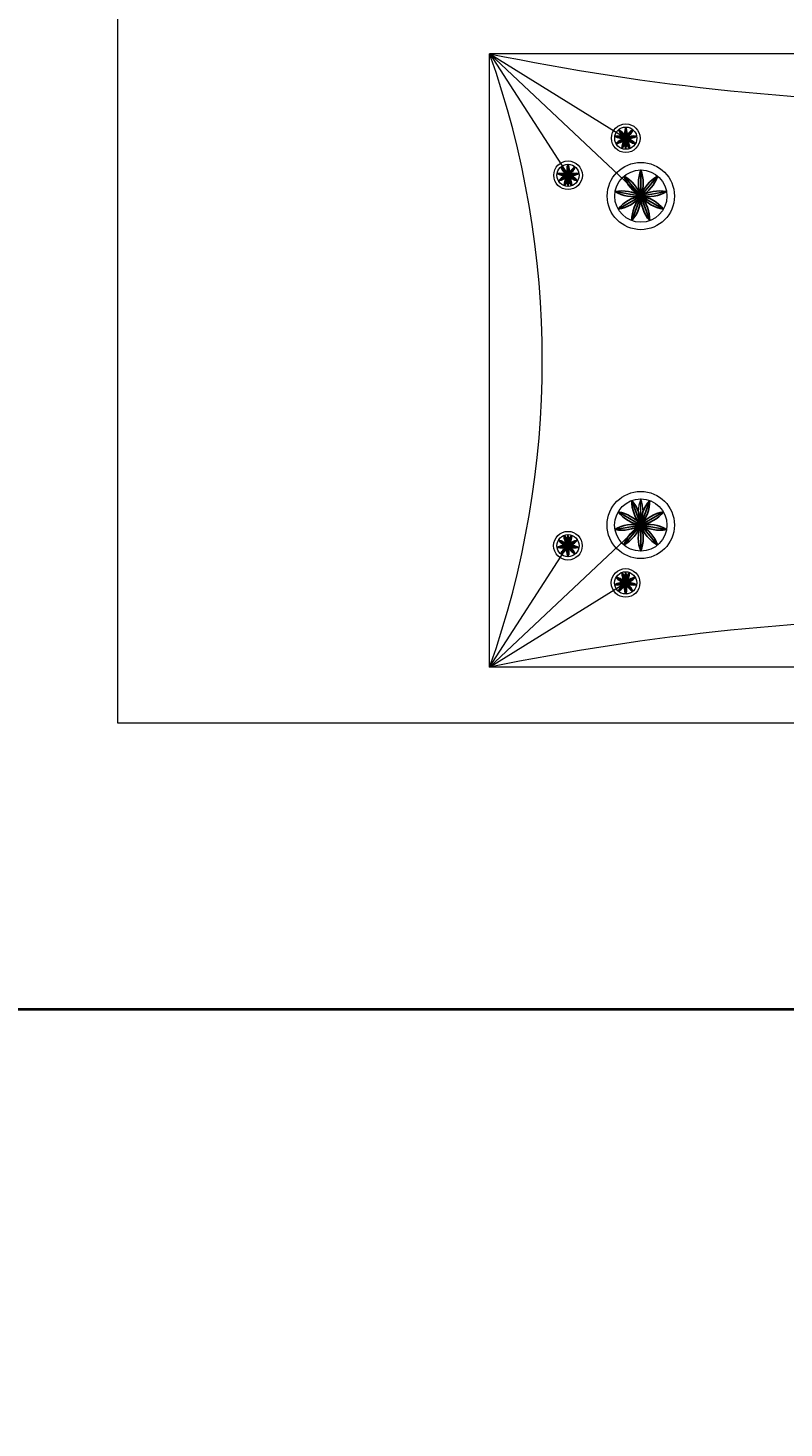
# Model space of a CAD drawing. Units: inches. Extents: x -46 to 1145, y -527 to 760.
# Tile 25 of 57: x 47 to 63, y 222 to 252. Entities that reach past the tile are written whole.
import ezdxf

# ---------------------------------------------------------------- set-up
doc = ezdxf.new("R2010")
doc.units = ezdxf.units.IN
doc.header["$MEASUREMENT"] = 0
for name, color, linetype, lineweight in [('A-ANNO-DIMS', 2, 'Continuous', 18), ('A-FURN', 2, 'Continuous', 13), ('WALLS', 4, 'Continuous', 40)]:
    doc.layers.add(name, color=color, linetype=linetype, lineweight=lineweight)
doc.layers.add('LT', color=9, linetype='Continuous')
doc.styles.get("Standard").update_dxf_attribs({"font": 'arial.ttf'})
doc.dimstyles.get("Standard").update_dxf_attribs({"dimtxt": 0.18, "dimasz": 0.18, "dimexe": 0.18, "dimexo": 0.0625, "dimgap": 0.09, "dimtad": 0, "dimtih": 1, "dimtoh": 1, "dimdec": 0, "dimzin": 0, "dimdsep": 46, "dimlunit": 3, "dimtxsty": 'Standard', "dimcen": 0.09, "dimadec": 0, "dimazin": 0, "dimtfac": 1, "dimtdec": 0, "dimtofl": 0, "dimtmove": 0, "dimatfit": 3, "dimfxl": 1, "dimtolj": 1, "dimtzin": 0, "dimarcsym": 0})

# ---------------------------------------------------------------- blocks, each defined once
blk = doc.blocks.new('*U58')
at = {"layer": 'LT'}
blk.add_line((0, 0.281), (0, -0.281), dxfattribs=at)
for centre, start, end in [((0.734, 0), 159.0676, 200.9324), ((-0.734, 0), 339.0676, 20.9324)]:
    blk.add_arc(centre, 0.786, start, end, dxfattribs=at)
blk = doc.blocks.new('*U59')
at = {"layer": 'LT', "transparency": 16777216}
blk.add_blockref('*U58', (609.936, 444.026), dxfattribs=at)
for p, rotation in [((609.756, 443.96), 40.00000000000002), ((610.117, 443.96), 320), ((609.659, 443.794), 80.00000000000001), ((609.693, 443.605), 120), ((609.84, 443.481), 160), ((610.032, 443.481), 200), ((610.179, 443.605), 240), ((610.213, 443.794), 280)]:
    blk.add_blockref('*U58', p, dxfattribs=dict(at, rotation=rotation))
blk = doc.blocks.new('*U60')
at = {"layer": 'LT'}
blk.add_line((0, 0.12), (0, -0.12), dxfattribs=at)
for centre, start, end in [((0.313, 0), 159.0676, 200.9324), ((-0.313, 0), 339.0676, 20.9324)]:
    blk.add_arc(centre, 0.335, start, end, dxfattribs=at)
blk = doc.blocks.new('*U61')
at = {"layer": 'LT', "transparency": 16777216}
for p, rotation in [((259.495, 188.896), 80.00000000000001), ((259.509, 188.816), 120), ((259.536, 188.967), 40), ((259.572, 188.763), 160), ((259.654, 188.763), 200), ((259.69, 188.967), 320), ((259.716, 188.816), 240), ((259.731, 188.896), 280)]:
    blk.add_blockref('*U60', p, dxfattribs=dict(at, rotation=rotation))
blk.add_blockref('*U60', (259.613, 188.995), dxfattribs=at)
blk = doc.blocks.new('*U62')
at = {"layer": 'LT'}
blk.add_line((0, 0.12), (0, -0.12), dxfattribs=at)
for centre, start, end in [((0.313, 0), 159.0676, 200.9324), ((-0.313, 0), 339.0676, 20.9324)]:
    blk.add_arc(centre, 0.335, start, end, dxfattribs=at)
blk = doc.blocks.new('*U63')
at = {"layer": 'LT', "transparency": 16777216}
for p, rotation in [((259.495, 188.896), 80.00000000000001), ((259.509, 188.816), 120), ((259.536, 188.967), 40), ((259.572, 188.763), 160), ((259.654, 188.763), 200), ((259.69, 188.967), 320), ((259.716, 188.816), 240), ((259.731, 188.896), 280)]:
    blk.add_blockref('*U62', p, dxfattribs=dict(at, rotation=rotation))
blk.add_blockref('*U62', (259.613, 188.995), dxfattribs=at)
blk = doc.blocks.new('*U70')
at = {"layer": 'LT'}
blk.add_line((0, 0.281), (0, -0.281), dxfattribs=at)
for centre, start, end in [((0.734, 0), 159.0676, 200.9324), ((-0.734, 0), 339.0676, 20.9324)]:
    blk.add_arc(centre, 0.786, start, end, dxfattribs=at)
blk = doc.blocks.new('*U71')
at = {"layer": 'LT', "transparency": 16777216}
blk.add_blockref('*U70', (609.936, 444.026), dxfattribs=at)
for p, rotation in [((609.756, 443.96), 40.00000000000002), ((610.117, 443.96), 320), ((609.659, 443.794), 80.00000000000001), ((609.693, 443.605), 120), ((609.84, 443.481), 160), ((610.032, 443.481), 200), ((610.179, 443.605), 240), ((610.213, 443.794), 280)]:
    blk.add_blockref('*U70', p, dxfattribs=dict(at, rotation=rotation))
blk = doc.blocks.new('*U46')
at = {"layer": 'LT'}
blk.add_line((0, 0.12), (0, -0.12), dxfattribs=at)
for centre, start, end in [((0.313, 0), 159.0676, 200.9324), ((-0.313, 0), 339.0676, 20.9324)]:
    blk.add_arc(centre, 0.335, start, end, dxfattribs=at)
blk = doc.blocks.new('*U47')
at = {"layer": 'LT', "transparency": 16777216}
for p, rotation in [((259.495, 188.896), 80.00000000000001), ((259.509, 188.816), 120), ((259.536, 188.967), 40), ((259.572, 188.763), 160), ((259.654, 188.763), 200), ((259.69, 188.967), 320), ((259.716, 188.816), 240), ((259.731, 188.896), 280)]:
    blk.add_blockref('*U46', p, dxfattribs=dict(at, rotation=rotation))
blk.add_blockref('*U46', (259.613, 188.995), dxfattribs=at)
blk = doc.blocks.new('*U48')
at = {"layer": 'LT'}
blk.add_line((0, 0.12), (0, -0.12), dxfattribs=at)
for centre, start, end in [((0.313, 0), 159.0676, 200.9324), ((-0.313, 0), 339.0676, 20.9324)]:
    blk.add_arc(centre, 0.335, start, end, dxfattribs=at)
blk = doc.blocks.new('*U49')
at = {"layer": 'LT', "transparency": 16777216}
for p, rotation in [((259.495, 188.896), 80.00000000000001), ((259.509, 188.816), 120), ((259.536, 188.967), 40), ((259.572, 188.763), 160), ((259.654, 188.763), 200), ((259.69, 188.967), 320), ((259.716, 188.816), 240), ((259.731, 188.896), 280)]:
    blk.add_blockref('*U48', p, dxfattribs=dict(at, rotation=rotation))
blk.add_blockref('*U48', (259.613, 188.995), dxfattribs=at)
blk = doc.blocks.new('BED-QUEEN-FURNISHED')
for p, q in [((0, 80), (60, 80)), ((60, 80), (60, 0)), ((31.2, 78.8), (52, 78.8)), ((31.2, 78.8), (52, 78.8)), ((52, 78.8), (48.615, 75.613)), ((52, 78.8), (49.074, 76.984)), ((52, 78.8), (50.315, 76.184)), ((52, 78.8), (52, 65.6)), ((52, 78.8), (52, 65.6)), ((49.074, 76.984), (49.074, 76.745)), ((50.315, 76.184), (50.315, 75.945)), ((48.748, 75.739), (48.748, 75.177)), ((51.995, 65.6), (48.612, 68.789)), ((50.312, 68.216), (50.313, 68.456)), ((51.995, 65.6), (50.312, 68.216)), ((49.07, 67.418), (49.07, 67.657)), ((51.995, 65.6), (49.07, 67.418)), ((31.2, 65.6), (52, 65.6)), ((31.2, 65.6), (52, 65.6))]:
    blk.add_line(p, q)
for centre, radius in [((49.074, 76.984), 0.308), ((49.074, 76.984), 0.239), ((48.748, 75.739), 0.723), ((48.748, 75.739), 0.562), ((50.315, 76.184), 0.308), ((50.315, 76.184), 0.239), ((48.746, 68.663), 0.723), ((48.746, 68.663), 0.562), ((50.312, 68.216), 0.308), ((50.312, 68.216), 0.239), ((49.07, 67.418), 0.308), ((49.07, 67.418), 0.239)]:
    blk.add_circle(centre, radius)
for centre, radius, start, end in [((41.6, 129.177), 51.439, 258.3356, 281.6644), ((70.653, 72.2), 19.787, 160.5151, 199.4849), ((49.386, 76.865), 0.335, 159.0676, 200.9324), ((48.761, 76.865), 0.335, 339.0676, 20.9324), ((50.628, 76.065), 0.335, 159.0676, 200.9324), ((50.003, 76.065), 0.335, 339.0676, 20.9324), ((49.483, 75.458), 0.786, 159.0676, 200.9324), ((48.014, 75.458), 0.786, 339.0676, 20.9324), ((50.625, 68.336), 0.335, 159.028, 200.8928), ((50, 68.336), 0.335, 339.028, 20.8928), ((49.383, 67.537), 0.335, 159.028, 200.8928), ((48.758, 67.537), 0.335, 339.028, 20.8928), ((41.6, 15.223), 51.439, 78.3356, 101.6644)]:
    blk.add_arc(centre, radius, start, end)
for name, p in [('*U63', (-210.539, -111.891)), ('*U59', (-561.188, -368.006)), ('*U61', (-209.298, -112.691))]:
    blk.add_blockref(name, p)
at = {"xscale": -1, "rotation": 179.9603994254766}
for name, p in [('*U71', (-560.883, 512.83)), ('*U47', (-209.17, 257.271)), ('*U49', (-210.412, 256.472))]:
    blk.add_blockref(name, p, dxfattribs=at)
blk = doc.blocks.new('*D685')
at = {"layer": 'A-ANNO-DIMS', "color": 0, "lineweight": -2, "transparency": 16777216}
for p, q in [((183.501, 700.889), (-46.216, 700.889)), ((-46.036, 700.709), (-46.036, 116.385)), ((-46.036, -468.302), (-46.036, 116.021)), ((12.501, -468.482), (-46.216, -468.482))]:
    blk.add_line(p, q, dxfattribs=at)
at = {"layer": 'A-ANNO-DIMS', "color": 0, "transparency": 16777216}
for points in [[(-46.066, 700.709), (-46.006, 700.709), (-46.036, 700.889)], [(-46.066, -468.302), (-46.006, -468.302), (-46.036, -468.482)]]:
    blk.add_solid(points, dxfattribs=at)
at = {"layer": 'Defpoints', "color": 0, "transparency": 16777216}
for p in [(-46.036, 700.889), (183.564, 700.889), (12.564, -468.482)]:
    blk.add_point(p, dxfattribs=at)
at = {"layer": 'A-ANNO-DIMS', "color": 0, "transparency": 16777216, "insert": (-46.036, 116.203), "char_height": 0.18, "attachment_point": 5}
blk.add_mtext('\\A1;1169.4', dxfattribs=at)

msp = doc.modelspace()

# ---------------------------------------------------------------- linework, layer by layer
at = {"layer": 'WALLS'}
msp.add_line((183.5637, 230.5176), (21.5637, 230.5176), dxfattribs=at)

# ---------------------------------------------------------------- block references
at = {"layer": 'A-FURN', "rotation": 180}
msp.add_blockref('BED-QUEEN-FURNISHED', (108.4877, 316.6818), dxfattribs=at)

# ---------------------------------------------------------------- dimensions: what is measured, and where the dimension line sits
at = {"layer": 'A-ANNO-DIMS'}
dim = msp.add_linear_dim(base=(-46.0363, 700.8886), p1=(12.5637, -468.4824), p2=(183.5637, 700.8886), angle=90, dimstyle='Standard', override={"dimdec": 1, "dimlfac": 1, "dimrnd": 0, "dimzin": 0, "dimdsep": 46, "dimlunit": 2}, dxfattribs=at)
dim.commit()
dim.dimension.update_dxf_attribs({"geometry": '*D685', "text_midpoint": (-46.0363, 116.2031)})

doc.saveas('drawing.dxf')
